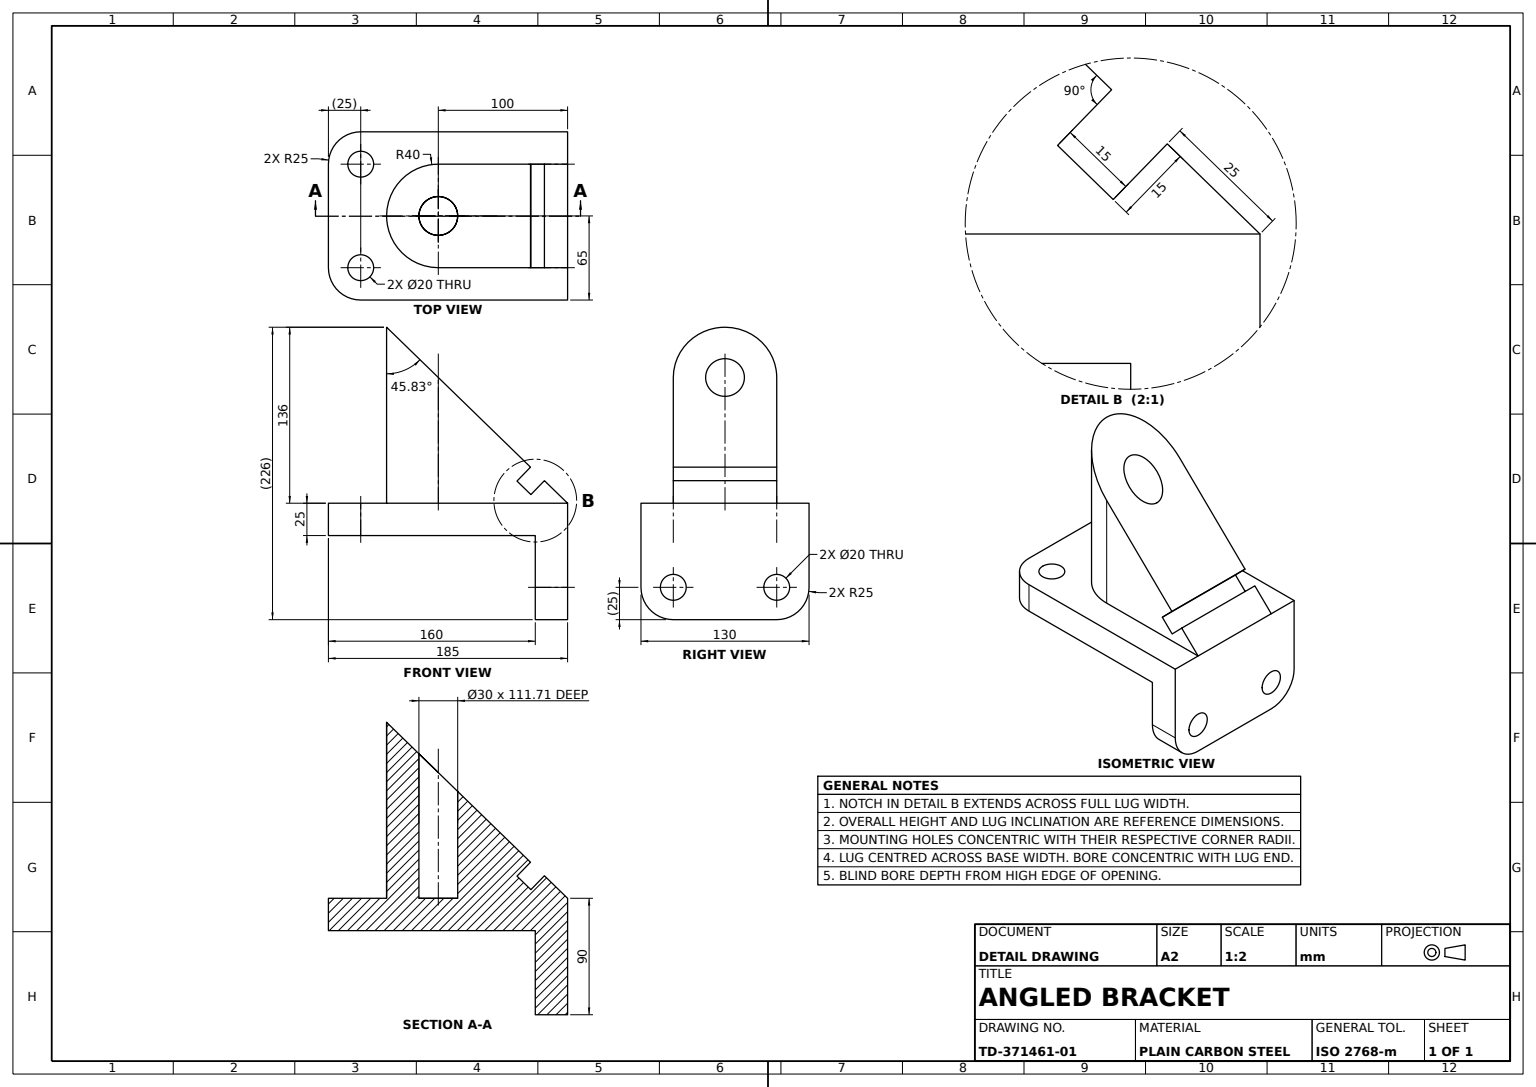
SolidWorks part; units mm, degrees
material "Plain Carbon Steel"
ref_plane "Front Plane" through (0, 0, 0) normal (0, 0, 1) x (1, 0, 0)
ref_plane "Top Plane" through (0, 0, 0) normal (0, 1, 0) x (1, 0, 0)
ref_plane "Right Plane" through (0, 0, 0) normal (1, 0, 0) x (0, 0, -1)
sketch "Base Plate Sketch" plane through (0, 0, 0) normal (0, 0, 1) x (1, 0, 0)
  line L1 (-69.8954, 0) -> (60.1046, 0)
  line L2 (-69.8954, 0) -> (-69.8954, -65)
  line L3 (-44.8954, -90) -> (35.1046, -90)
  line L4 (60.1046, 0) -> (60.1046, -65)
  arc A0 (35.1046, -90) -> (60.1046, -65) centre (35.1046, -65) ccw
  arc A1 (-69.8954, -65) -> (-44.8954, -90) centre (-44.8954, -65) ccw
  circle A2 centre (-44.8954, -65) radius 10
  circle A3 centre (35.1046, -65) radius 10
  point P6 (60.1046, -90)
  dimension "D3" = 25
  dimension "D4" = 20
  dimension "D5" = 20
  dimension "D1" = 130
  dimension "D2" = 90
  dimension "D6" = 69.8954
extrude "Base Plate" add sketch "Base Plate Sketch" along normal blind 25
sketch "Flange Sketch" plane through (0, 0, 0) normal (0, 0, -1) x (-1, 0, 0)
  line L0 (69.8954, 0) -> (69.8954, -65) construction
  line L1 (-60.1046, 0) -> (69.8954, 0)
  line L2 (-60.1046, 0) -> (-60.1046, -25)
  line L3 (-60.1046, -25) -> (69.8954, -25)
  line L4 (69.8954, 0) -> (69.8954, -25)
  dimension "D1" = 25
extrude "Flange" add sketch "Flange Sketch" along normal blind 160
sketch "Flange Profile Cut Sketch" plane through (0, 0, 0) normal (0, 1, 0) x (1, 0, 0)
  line L0 (60.1046, -25) -> (60.1046, 160) construction
  line L1 (-44.8954, 160) -> (35.1046, 160)
  line L2 (-69.8954, 135) -> (-69.8954, 0)
  line L3 (-69.8954, 0) -> (60.1046, 0)
  line L4 (60.1046, 135) -> (60.1046, 0)
  line L5 (-69.8954, 135) -> (-69.8954, 160)
  line L6 (-69.8954, 160) -> (-44.8954, 160)
  line L7 (60.1046, 135) -> (60.1046, 160)
  line L8 (60.1046, 160) -> (35.1046, 160)
  arc A0 (35.1046, 160) -> (60.1046, 135) centre (35.1046, 135) cw
  arc A1 (-44.8954, 160) -> (-69.8954, 135) centre (-44.8954, 135) ccw
  point P11 (-69.8954, 160)
  line M7 (60.1046, -25) -> (60.1046, 160)
  line M8 (60.1046, 160) -> (-69.8954, 160)
  line M9 (-69.8954, 160) -> (-69.8954, -25)
  dimension "D1" = 25
  dimension "D2" = 25
extrude "Flange Profile Cut" cut sketch "Flange Profile Cut Sketch" against normal blind 160 contours A0 M8 M7 | A1 M8 M9
sketch "Holes Sketch" plane through (0, 0, 0) normal (0, 1, 0) x (1, 0, 0)
  circle A0 centre (-44.8954, 135) radius 10
  circle A1 centre (35.1046, 135) radius 10
  dimension "D1" = 20
  dimension "D2" = 20
extrude "Holes Cut" cut sketch "Holes Sketch" against normal blind 160
sketch "Lug Sketch" plane through (0, 0, 0) normal (0, 1, 0) x (1, 0, 0)
  line L1 (-44.8954, -25) -> (35.1046, -25)
  line L2 (-44.8954, -25) -> (-44.8954, 75)
  line L4 (35.1046, -25) -> (35.1046, 75)
  arc A0 (-44.8954, 75) -> (35.1046, 75) centre (-4.8954, 75) cw
  circle A1 centre (-4.8954, 75) radius 15
  dimension "D4" = 30
  dimension "D1" = 80
  dimension "D2" = 100
extrude "Lug" add sketch "Lug Sketch" along normal blind 136
sketch "Lug 45deg Trim Sketch" plane through (35.1046, 0, 0) normal (1, 0, 0) x (0, 0, -1)
  line L1 (-25, 0) -> (75, 0) construction
  line L2 (-25, 0) -> (135, 0) construction
  line L3 (46.0145, 68.9855) -> (45, 70)
  line L4 (-25, 0) -> (-25, 136)
  line L5 (-25, 136) -> (115, 136)
  line L6 (115, 136) -> (75, 136) construction
  line L7 (115, 136) -> (115, 0)
  line L8 (-25, 0) -> (115, 136)
  line L9 (75, 136) -> (75, 0) construction
  dimension "D1" = 45
  dimension "D2" = 30
extrude "Lug 45deg Trim" cut sketch "Lug 45deg Trim Sketch" against normal blind 136
sketch "Lug Notch Sketch" plane through (35.1046, 0, 0) normal (1, 0, 0) x (0, 0, -1)
  line L0 (-7.068, 17.4196) -> (3.6912, 27.8714)
  line L1 (-7.068, 17.4196) -> (3.3838, 6.6605)
  line L2 (3.6912, 27.8714) -> (14.143, 17.1122)
  line L3 (3.3838, 6.6605) -> (14.143, 17.1122)
  line L4 (-25, 0) -> (75, 97.1429) construction
  dimension "D1" = 25
  dimension "D2" = 15
  dimension "D3" = 15
extrude "Lug Notch" cut sketch "Lug Notch Sketch" against normal blind 136
